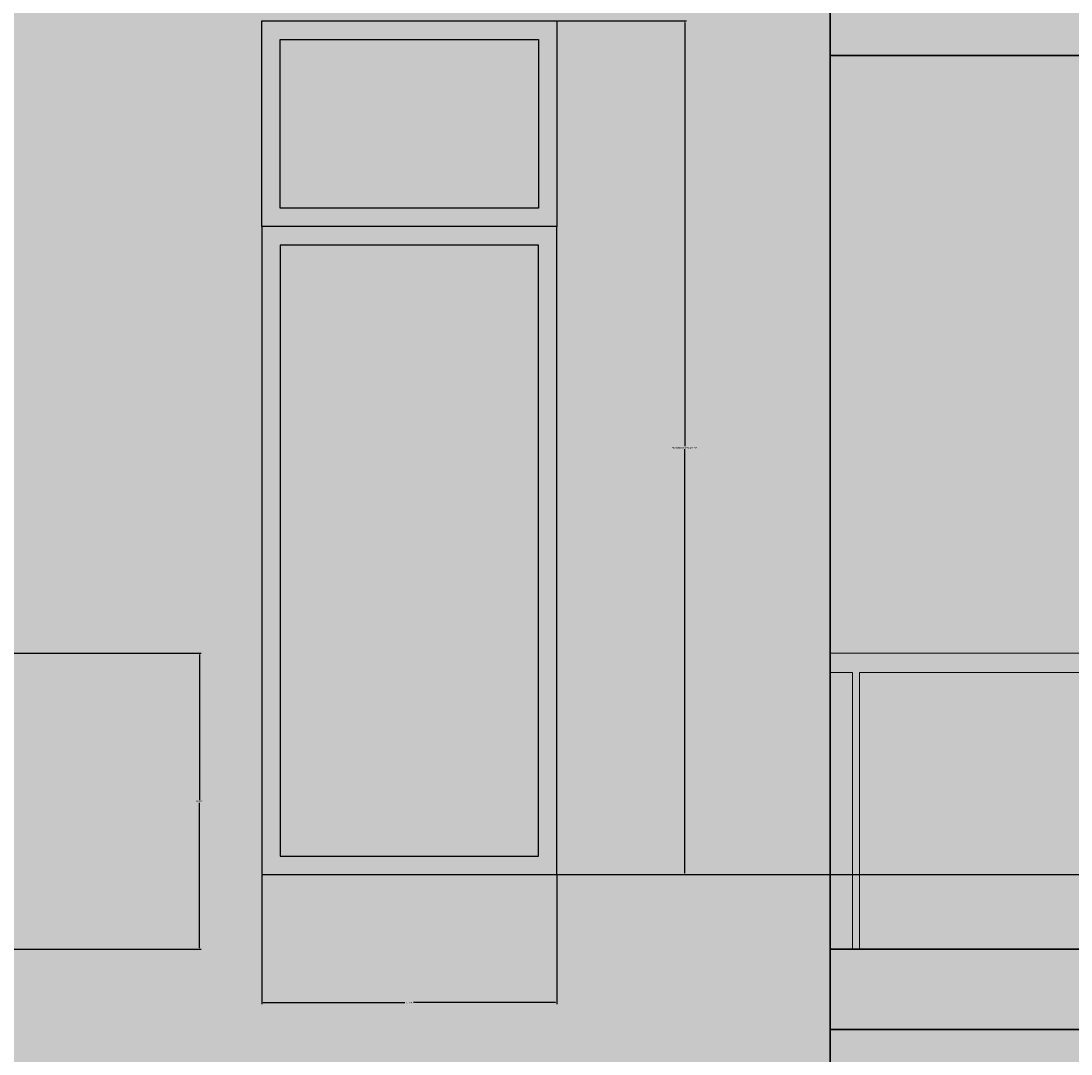
# Model space of a CAD drawing. Units: feet. Extents: x 2893 to 4112, y 897 to 1573.
# Tile 3 of 7: x 3123 to 3253, y 1090 to 1217. Entities that reach past the tile are written whole.
import ezdxf

# ---------------------------------------------------------------- set-up
doc = ezdxf.new("R2010")
doc.units = ezdxf.units.FT
for name, color, linetype, lineweight in [('A-ANNO-DIMS', 2, 'Continuous', 18), ('A-ELEV', 7, 'Continuous', 35), ('A-ELEV-PATT', 8, 'Continuous', 13), ('A-ELEV-RAIL', 4, 'Continuous', 18), ('A-GLAZ', 4, 'Continuous', 25)]:
    doc.layers.add(name, color=color, linetype=linetype, lineweight=lineweight)
doc.styles.get("Standard").update_dxf_attribs({"font": 'arial.ttf'})
doc.dimstyles.get("Standard").update_dxf_attribs({"dimtxt": 0.18, "dimasz": 0.18, "dimexe": 0.18, "dimexo": 0.0625, "dimgap": 0.09, "dimtad": 0, "dimtih": 1, "dimtoh": 1, "dimdec": 1, "dimzin": 0, "dimdsep": 46, "dimlunit": 3, "dimtxsty": 'Standard', "dimcen": 0.09, "dimadec": 0, "dimazin": 0, "dimtfac": 1, "dimtdec": 1, "dimtofl": 0, "dimtmove": 0, "dimatfit": 3, "dimfxl": 1, "dimtolj": 1, "dimtzin": 0, "dimarcsym": 0})

# ---------------------------------------------------------------- blocks, each defined once
blk = doc.blocks.new('WIN-FEATURE')
for points in [[(36.35, 79.81), (0, 79.81), (0, 105.14), (36.35, 105.14)], [(36.35, 79.81), (0, 79.81), (0, 105.14), (36.35, 105.14)], [(34.08, 82.08), (2.27, 82.08), (2.27, 102.87), (34.08, 102.87)], [(34.08, 82.08), (2.27, 82.08), (2.27, 102.87), (34.08, 102.87)], [(0, 0), (36.35, 0), (36.35, 79.81), (0, 79.81)], [(0, 0), (36.35, 0), (36.35, 79.81), (0, 79.81)], [(2.27, 2.27), (34.08, 2.27), (34.08, 77.54), (2.27, 77.54)], [(2.27, 2.27), (34.08, 2.27), (34.08, 77.54), (2.27, 77.54)]]:
    blk.add_lwpolyline(points, close=True)
blk = doc.blocks.new('BALCONY-RAIL')
blk.add_lwpolyline([(56.56, 34.07), (3.3, 34.07), (3.3, 0), (2.43, 0), (2.43, 34.07), (0, 34.07), (0, 36.45), (173.25, 36.45), (173.25, 34.07), (170.48, 34.07), (170.48, 0), (169.61, 0), (169.61, 34.07), (115.47, 34.07), (115.47, 0), (114.59, 0), (114.59, 34.07), (57.43, 34.07), (57.43, 0), (56.56, 0)], close=True)
blk.add_lwpolyline([(56.56, 34.07), (3.3, 34.07), (3.3, 0), (2.43, 0), (2.43, 34.07), (0, 34.07), (0, 36.45), (173.25, 36.45), (173.25, 34.07), (170.48, 34.07), (170.48, 0), (169.61, 0), (169.61, 34.07), (115.47, 34.07), (115.47, 0), (114.59, 0), (114.59, 34.07), (57.43, 34.07), (57.43, 0), (56.56, 0)], close=True)
blk = doc.blocks.new('*D8')
at = {"layer": 'A-ANNO-DIMS', "color": 0, "lineweight": -2, "transparency": 16777216}
for p, q in [((3119.39, 1139.38), (3145.49, 1139.38)), ((3145.31, 1139.2), (3145.31, 1121.34)), ((3145.31, 1103.11), (3145.31, 1120.97)), ((3119.39, 1102.93), (3145.49, 1102.93))]:
    blk.add_line(p, q, dxfattribs=at)
at = {"layer": 'A-ANNO-DIMS', "color": 0, "transparency": 16777216}
for points in [[(3145.28, 1139.2), (3145.34, 1139.2), (3145.31, 1139.38)], [(3145.28, 1103.11), (3145.34, 1103.11), (3145.31, 1102.93)]]:
    blk.add_solid(points, dxfattribs=at)
at = {"layer": 'Defpoints', "color": 0, "transparency": 16777216}
for p in [(3119.33, 1139.38), (3145.31, 1139.38), (3119.33, 1102.93)]:
    blk.add_point(p, dxfattribs=at)
at = {"layer": 'A-ANNO-DIMS', "color": 0, "transparency": 16777216, "insert": (3145.31, 1121.16), "char_height": 0.18, "attachment_point": 5}
blk.add_mtext('\\A1;36 TYP.', dxfattribs=at)
blk = doc.blocks.new('*D9')
at = {"layer": 'A-ANNO-DIMS', "color": 0, "lineweight": -2, "transparency": 16777216}
for p, q in [((3189.38, 1217.25), (3205.27, 1217.25)), ((3205.09, 1217.07), (3205.09, 1164.86)), ((3205.09, 1112.29), (3205.09, 1164.5)), ((3189.38, 1112.11), (3205.27, 1112.11))]:
    blk.add_line(p, q, dxfattribs=at)
at = {"layer": 'A-ANNO-DIMS', "color": 0, "transparency": 16777216}
for points in [[(3205.06, 1217.07), (3205.12, 1217.07), (3205.09, 1217.25)], [(3205.06, 1112.29), (3205.12, 1112.29), (3205.09, 1112.11)]]:
    blk.add_solid(points, dxfattribs=at)
at = {"layer": 'Defpoints', "color": 0, "transparency": 16777216}
for p in [(3189.32, 1217.25), (3205.09, 1217.25), (3189.32, 1112.11)]:
    blk.add_point(p, dxfattribs=at)
at = {"layer": 'A-ANNO-DIMS', "color": 0, "transparency": 16777216, "insert": (3205.09, 1164.68), "char_height": 0.18, "attachment_point": 5}
blk.add_mtext('\\A1;FEATURE WINDOW 105 TYP.', dxfattribs=at)
blk = doc.blocks.new('*D10')
at = {"layer": 'A-ANNO-DIMS', "color": 0, "lineweight": -2, "transparency": 16777216}
for p, q in [((3152.97, 1112.05), (3152.97, 1096.16)), ((3189.32, 1112.05), (3189.32, 1096.16)), ((3153.15, 1096.34), (3170.61, 1096.34)), ((3189.14, 1096.34), (3171.67, 1096.34))]:
    blk.add_line(p, q, dxfattribs=at)
at = {"layer": 'A-ANNO-DIMS', "color": 0, "transparency": 16777216}
for points in [[(3153.15, 1096.37), (3153.15, 1096.31), (3152.97, 1096.34)], [(3189.14, 1096.37), (3189.14, 1096.31), (3189.32, 1096.34)]]:
    blk.add_solid(points, dxfattribs=at)
at = {"layer": 'Defpoints', "color": 0, "transparency": 16777216}
for p in [(3152.97, 1112.11), (3189.32, 1112.11), (3189.32, 1096.34)]:
    blk.add_point(p, dxfattribs=at)
at = {"layer": 'A-ANNO-DIMS', "color": 0, "transparency": 16777216, "insert": (3171.14, 1096.34), "char_height": 0.18, "attachment_point": 5}
blk.add_mtext('\\A1;36 TYP.', dxfattribs=at)
blk = doc.blocks.new('*D48')
at = {"layer": 'A-ANNO-DIMS', "color": 0, "lineweight": -2, "transparency": 16777216}
for p, q in [((2924.72, 1491.83), (2924.72, 897.37)), ((3417.56, 1491.83), (3417.56, 897.37)), ((2924.9, 897.55), (3170.74, 897.55)), ((3417.38, 897.55), (3171.54, 897.55))]:
    blk.add_line(p, q, dxfattribs=at)
at = {"layer": 'A-ANNO-DIMS', "color": 0, "transparency": 16777216}
for points in [[(2924.9, 897.58), (2924.9, 897.52), (2924.72, 897.55)], [(3417.38, 897.58), (3417.38, 897.52), (3417.56, 897.55)]]:
    blk.add_solid(points, dxfattribs=at)
at = {"layer": 'Defpoints', "color": 0, "transparency": 16777216}
for p in [(2924.72, 1491.89), (3417.56, 1491.89), (3417.56, 897.55)]:
    blk.add_point(p, dxfattribs=at)
at = {"layer": 'A-ANNO-DIMS', "color": 0, "transparency": 16777216, "insert": (3171.14, 897.55), "char_height": 0.18, "attachment_point": 5}
blk.add_mtext('\\A1;492.8', dxfattribs=at)
blk = doc.blocks.new('*D51')
at = {"layer": 'A-ANNO-DIMS', "color": 0, "lineweight": -2, "transparency": 16777216}
for p, q in [((3189.38, 1112.11), (3449.24, 1112.11)), ((3449.06, 1111.93), (3449.06, 1099.74)), ((3449.06, 1087.19), (3449.06, 1099.38)), ((3215.03, 1087.01), (3449.24, 1087.01))]:
    blk.add_line(p, q, dxfattribs=at)
at = {"layer": 'A-ANNO-DIMS', "color": 0, "transparency": 16777216}
for points in [[(3449.03, 1111.93), (3449.09, 1111.93), (3449.06, 1112.11)], [(3449.03, 1087.19), (3449.09, 1087.19), (3449.06, 1087.01)]]:
    blk.add_solid(points, dxfattribs=at)
at = {"layer": 'Defpoints', "color": 0, "transparency": 16777216}
for p in [(3189.32, 1112.11), (3449.06, 1112.11), (3214.97, 1087.01)]:
    blk.add_point(p, dxfattribs=at)
at = {"layer": 'A-ANNO-DIMS', "color": 0, "transparency": 16777216, "insert": (3449.06, 1099.56), "char_height": 0.18, "attachment_point": 5}
blk.add_mtext('\\A1;25.095', dxfattribs=at)

msp = doc.modelspace()

# ---------------------------------------------------------------- hatches: boundary and pattern name
at = {"layer": 'A-ELEV-PATT'}
h = msp.add_hatch(color=256, dxfattribs=at)
h.dxf.hatch_style = 1
h.paths.add_polyline_path([(3222.9589, 1541.1646), (3119.3255, 1541.1646), (3119.3255, 967.0143), (3127.3151, 967.0143), (3127.3151, 1087.0143), (3214.9693, 1087.0143), (3214.9693, 1078.6766), (3214.9693, 967.0143), (3222.9589, 967.0143)])
h.paths.add_polyline_path([(3152.9675, 1482.3616), (3189.3169, 1482.3616), (3189.3169, 1457.0324), (3189.3169, 1377.2236), (3152.9675, 1377.2236), (3152.9675, 1457.0324)], flags=16)
h.paths.add_polyline_path([(3155.237, 1480.0922), (3187.0474, 1480.0922), (3187.0474, 1459.3019), (3155.237, 1459.3019)], flags=0)
h.paths.add_polyline_path([(3155.237, 1454.7629), (3187.0474, 1454.7629), (3187.0474, 1379.4931), (3155.237, 1379.4931)], flags=0)
h.paths.add_polyline_path([(3152.9675, 1354.8437), (3189.3169, 1354.8437), (3189.3169, 1329.5145), (3189.3169, 1249.7057), (3152.9675, 1249.7057), (3152.9675, 1329.5145)], flags=16)
h.paths.add_polyline_path([(3155.237, 1352.5742), (3187.0474, 1352.5742), (3187.0474, 1331.784), (3155.237, 1331.784)], flags=0)
h.paths.add_polyline_path([(3155.237, 1327.245), (3187.0474, 1327.245), (3187.0474, 1251.9752), (3155.237, 1251.9752)], flags=0)
h.paths.add_polyline_path([(3152.9675, 1217.2478), (3189.3169, 1217.2478), (3189.3169, 1191.9186), (3189.3169, 1112.1098), (3152.9675, 1112.1098), (3152.9675, 1191.9186)], flags=16)
h.paths.add_polyline_path([(3155.237, 1214.9783), (3187.0474, 1214.9783), (3187.0474, 1194.1881), (3155.237, 1194.1881)], flags=0)
h.paths.add_polyline_path([(3155.237, 1189.6491), (3187.0474, 1189.6491), (3187.0474, 1114.3793), (3155.237, 1114.3793)], flags=0)
h = msp.add_hatch(dxfattribs=at)
h.set_pattern_fill('AR-BRELM', color=256, scale=0.1)
h.set_pattern_definition([(0, (-663.002, 0), (0, 13.5484), [19.3675, -0.9525]), (0, (-663.002, 5.715), (0, 13.5484), [19.3675, -0.9525]), (0, (-657.922, 6.774), (0, 13.5484), [9.2075, -0.9525]), (0, (-657.922, 12.489), (0, 13.5484), [9.2075, -0.9525]), (90, (-663.002, 0), (-20.32, 1e-15), [5.715, -7.8334]), (90, (-663.954, 0), (-20.32, 1e-15), [5.715, -7.8334]), (90, (-657.922, 6.774), (-10.16, 6e-16), [5.715, -7.8334]), (90, (-658.874, 6.774), (-10.16, 6e-16), [5.715, -7.8334])])
h.paths.add_polyline_path([(3222.9589, 1541.1646), (3119.3255, 1541.1646), (3119.3255, 967.0143), (3127.3151, 967.0143), (3127.3151, 1087.0143), (3214.9693, 1087.0143), (3214.9693, 1078.6766), (3214.9693, 967.0143), (3222.9589, 967.0143)])
h.paths.add_polyline_path([(3152.9675, 1482.3616), (3189.3169, 1482.3616), (3189.3169, 1457.0324), (3189.3169, 1377.2236), (3152.9675, 1377.2236), (3152.9675, 1457.0324)], flags=16)
h.paths.add_polyline_path([(3155.237, 1480.0922), (3187.0474, 1480.0922), (3187.0474, 1459.3019), (3155.237, 1459.3019)], flags=0)
h.paths.add_polyline_path([(3155.237, 1454.7629), (3187.0474, 1454.7629), (3187.0474, 1379.4931), (3155.237, 1379.4931)], flags=0)
h.paths.add_polyline_path([(3152.9675, 1354.8437), (3189.3169, 1354.8437), (3189.3169, 1329.5145), (3189.3169, 1249.7057), (3152.9675, 1249.7057), (3152.9675, 1329.5145)], flags=16)
h.paths.add_polyline_path([(3155.237, 1352.5742), (3187.0474, 1352.5742), (3187.0474, 1331.784), (3155.237, 1331.784)], flags=0)
h.paths.add_polyline_path([(3155.237, 1327.245), (3187.0474, 1327.245), (3187.0474, 1251.9752), (3155.237, 1251.9752)], flags=0)
h.paths.add_polyline_path([(3152.9675, 1217.2478), (3189.3169, 1217.2478), (3189.3169, 1191.9186), (3189.3169, 1112.1098), (3152.9675, 1112.1098), (3152.9675, 1191.9186)], flags=16)
h.paths.add_polyline_path([(3155.237, 1214.9783), (3187.0474, 1214.9783), (3187.0474, 1194.1881), (3155.237, 1194.1881)], flags=0)
h.paths.add_polyline_path([(3155.237, 1189.6491), (3187.0474, 1189.6491), (3187.0474, 1114.3793), (3155.237, 1114.3793)], flags=0)
h = msp.add_hatch(color=256, dxfattribs=at)
h.dxf.hatch_style = 1
h.paths.add_polyline_path([(3119.3255, 1527.889), (2924.7207, 1527.889), (2924.7207, 1491.889), (3119.3255, 1491.889)])
h.paths.add_polyline_path([(3417.5637, 1527.889), (3222.9589, 1527.889), (3222.9589, 1491.889), (3417.5637, 1491.889)])
h.paths.add_polyline_path([(3119.3255, 1102.9302), (2946.0771, 1102.9302), (2946.0771, 1139.3799), (2934.0287, 1139.3799), (2934.0287, 1093.0143), (3119.3255, 1093.0143)])
h.paths.add_polyline_path([(3119.3255, 1093.0143), (2934.4679, 1093.0143), (2934.4679, 1087.0143), (3119.3255, 1087.0143)])
h.paths.add_polyline_path([(3408.2557, 1139.3799), (3396.2073, 1139.3799), (3396.2073, 1136.9984), (3396.2073, 1102.9302), (3222.9589, 1102.9302), (3222.9589, 1093.0143), (3408.2557, 1093.0143)])
h.paths.add_polyline_path([(3407.8165, 1093.0143), (3222.9589, 1093.0143), (3222.9589, 1087.0143), (3407.8165, 1087.0143)])
h = msp.add_hatch(color=256, dxfattribs=at)
h.dxf.hatch_style = 1
h.paths.add_polyline_path([(3119.3255, 1491.889), (2924.7207, 1491.889), (2945.7801, 1471.0143), (3119.3255, 1471.0143)])
h.paths.add_polyline_path([(3119.3255, 1471.0143), (2945.7801, 1471.0143), (2951.8333, 1465.0143), (3119.3255, 1465.0143)])
h.paths.add_polyline_path([(3119.3255, 1465.0143), (2951.8333, 1465.0143), (2951.8333, 1381.4641), (2984.02, 1381.4641), (2984.02, 1432.3761), (3084.4999, 1432.3761), (3084.4999, 1381.4641), (3119.3255, 1381.4641)])
h.paths.add_polyline_path([(3417.5637, 1491.889), (3222.9589, 1491.889), (3222.9589, 1471.0143), (3396.5042, 1471.0143)])
h.paths.add_polyline_path([(3396.5042, 1471.0143), (3222.9589, 1471.0143), (3222.9589, 1465.0143), (3390.4511, 1465.0143)])
h.paths.add_polyline_path([(3390.4511, 1465.0143), (3222.9589, 1465.0143), (3222.9589, 1381.4641), (3257.7845, 1381.4641), (3257.7845, 1432.3761), (3358.2644, 1432.3761), (3358.2644, 1381.4641), (3390.4511, 1381.4641)])
h.paths.add_polyline_path([(3119.3255, 1339.0143), (2942.6825, 1339.0143), (2942.6825, 1232.1197), (2948.5078, 1232.1197), (2948.5078, 1266.188), (2946.0771, 1266.188), (2946.0771, 1268.5695), (2984.02, 1268.5695), (2984.02, 1319.4815), (3084.4999, 1319.4815), (3084.4999, 1268.5695), (3119.3255, 1268.5695)], flags=17)
h.paths.add_polyline_path([(3399.6019, 1339.0143), (3222.9589, 1339.0143), (3222.9589, 1268.5695), (3257.7845, 1268.5695), (3257.7845, 1319.4815), (3358.2644, 1319.4815), (3358.2644, 1268.5695), (3396.2073, 1268.5695), (3396.2073, 1266.188), (3393.7766, 1266.188), (3393.7766, 1232.1197), (3399.6019, 1232.1197)], flags=17)
h.paths.add_polyline_path([(2942.6825, 1339.0143), (3119.3255, 1339.0143), (3119.3255, 1345.0143), (2933.3946, 1345.0143), (2933.3946, 1232.1197), (2933.3946, 1220.0947), (3119.3255, 1220.0947), (3119.3255, 1232.1197), (2942.6825, 1232.1197)])
h.paths.add_polyline_path([(3408.8898, 1345.0143), (3222.9589, 1345.0143), (3222.9589, 1339.0143), (3399.6019, 1339.0143), (3399.6019, 1232.1197), (3393.7766, 1232.1197), (3392.9028, 1232.1197), (3222.9589, 1232.1197), (3222.9589, 1220.0947), (3408.8898, 1220.0947), (3408.8898, 1232.1197)])
h.paths.add_polyline_path([(2984.02, 1190.2919), (3084.4999, 1190.2919), (3084.4999, 1139.3799), (3119.3255, 1139.3799), (3119.3255, 1213.0143), (2951.8333, 1213.0143), (2951.8333, 1139.3799), (2984.02, 1139.3799)])
h.paths.add_polyline_path([(3119.3255, 1219.0143), (2934.0287, 1219.0143), (2951.8333, 1213.0143), (3119.3255, 1213.0143)])
h.paths.add_polyline_path([(3390.4511, 1213.0143), (3222.9589, 1213.0143), (3222.9589, 1139.3799), (3257.7845, 1139.3799), (3257.7845, 1190.2919), (3358.2644, 1190.2919), (3358.2644, 1139.3799), (3390.4511, 1139.3799)])
h.paths.add_polyline_path([(3408.2557, 1219.0143), (3222.9589, 1219.0143), (3222.9589, 1213.0143), (3408.2557, 1213.0143)])
h = msp.add_hatch(color=256, dxfattribs=at)
h.dxf.hatch_style = 1
h.paths.add_polyline_path([(3119.3255, 1139.3799), (2946.0771, 1139.3799), (2946.0771, 1136.9984), (2948.5078, 1136.9984), (2948.5078, 1102.9302), (2949.3816, 1102.9302), (2949.3816, 1136.9984), (3002.6337, 1136.9984), (3002.6337, 1102.9302), (3003.5075, 1102.9302), (3003.5075, 1136.9984), (3060.6708, 1136.9984), (3060.6708, 1102.9302), (3061.5445, 1102.9302), (3061.5445, 1136.9984), (3115.685, 1136.9984), (3115.685, 1102.9302), (3116.5588, 1102.9302), (3116.5588, 1136.9984), (3119.3255, 1136.9984)])
h.paths.add_polyline_path([(2987.1701, 1187.1419), (3033.6877, 1187.1419), (3033.6877, 1139.3799), (3034.8322, 1139.3799), (3034.8322, 1187.1419), (3081.3499, 1187.1419), (3081.3499, 1139.3799), (3084.4999, 1139.3799), (3084.4999, 1190.2919), (2984.02, 1190.2919), (2984.02, 1139.3799), (2987.1701, 1139.3799)])
h.paths.add_polyline_path([(2987.1701, 1316.3314), (3033.6877, 1316.3314), (3033.6877, 1268.5695), (3034.8322, 1268.5695), (3034.8322, 1316.3314), (3081.3499, 1316.3314), (3081.3499, 1268.5695), (3084.4999, 1268.5695), (3084.4999, 1319.4815), (2984.02, 1319.4815), (2984.02, 1268.5695), (2987.1701, 1268.5695)])
h.paths.add_polyline_path([(3003.5075, 1266.188), (3060.6708, 1266.188), (3060.6708, 1232.1197), (3061.5445, 1232.1197), (3061.5445, 1266.188), (3115.685, 1266.188), (3115.685, 1232.1197), (3116.5588, 1232.1197), (3116.5588, 1266.188), (3119.3255, 1266.188), (3119.3255, 1268.5695), (2946.0771, 1268.5695), (2946.0771, 1266.188), (2948.5078, 1266.188), (2948.5078, 1232.1197), (2949.3816, 1232.1197), (2949.3816, 1266.188), (3002.6337, 1266.188), (3002.6337, 1232.1197), (3003.5075, 1232.1197)])
h.paths.add_polyline_path([(2987.1701, 1429.226), (3033.6877, 1429.226), (3033.6877, 1381.4641), (3034.8322, 1381.4641), (3034.8322, 1429.226), (3081.3499, 1429.226), (3081.3499, 1381.4641), (3084.4999, 1381.4641), (3084.4999, 1432.3761), (2984.02, 1432.3761), (2984.02, 1381.4641), (2987.1701, 1381.4641)])
h.paths.add_polyline_path([(3119.3255, 1381.4641), (2946.0771, 1381.4641), (2946.0771, 1379.0826), (2948.5078, 1379.0826), (2948.5078, 1345.0143), (2949.3816, 1345.0143), (2949.3816, 1379.0826), (3002.6337, 1379.0826), (3002.6337, 1345.0143), (3003.5075, 1345.0143), (3003.5075, 1379.0826), (3060.6708, 1379.0826), (3060.6708, 1345.0143), (3061.5445, 1345.0143), (3061.5445, 1379.0826), (3115.685, 1379.0826), (3115.685, 1345.0143), (3116.5588, 1345.0143), (3116.5588, 1379.0826), (3119.3255, 1379.0826)])
h.paths.add_polyline_path([(3189.3169, 1482.3616), (3152.9675, 1482.3616), (3152.9675, 1457.0324), (3189.3169, 1457.0324)])
h.paths.add_polyline_path([(3155.237, 1480.0922), (3187.0474, 1480.0922), (3187.0474, 1459.3019), (3155.237, 1459.3019)], flags=16)
h.paths.add_polyline_path([(3189.3169, 1457.0324), (3152.9675, 1457.0324), (3152.9675, 1377.2236), (3189.3169, 1377.2236)])
h.paths.add_polyline_path([(3155.237, 1454.7629), (3187.0474, 1454.7629), (3187.0474, 1379.4931), (3155.237, 1379.4931)], flags=16)
h.paths.add_polyline_path([(3358.2644, 1432.3761), (3257.7845, 1432.3761), (3257.7845, 1381.4641), (3260.9345, 1381.4641), (3260.9345, 1429.226), (3307.4522, 1429.226), (3307.4522, 1381.4641), (3308.5967, 1381.4641), (3308.5967, 1429.226), (3355.1143, 1429.226), (3355.1143, 1381.4641), (3358.2644, 1381.4641)])
h.paths.add_polyline_path([(3396.2073, 1381.4641), (3222.9589, 1381.4641), (3222.9589, 1379.0826), (3225.7256, 1379.0826), (3225.7256, 1345.0143), (3226.5994, 1345.0143), (3226.5994, 1379.0826), (3280.7398, 1379.0826), (3280.7398, 1345.0143), (3281.6136, 1345.0143), (3281.6136, 1379.0826), (3338.7769, 1379.0826), (3338.7769, 1345.0143), (3339.6507, 1345.0143), (3339.6507, 1379.0826), (3392.9028, 1379.0826), (3392.9028, 1345.0143), (3393.7766, 1345.0143), (3393.7766, 1379.0826), (3396.2073, 1379.0826)])
h.paths.add_polyline_path([(3358.2644, 1319.4815), (3257.7845, 1319.4815), (3257.7845, 1268.5695), (3260.9345, 1268.5695), (3260.9345, 1316.3314), (3307.4522, 1316.3314), (3307.4522, 1268.5695), (3308.5967, 1268.5695), (3308.5967, 1316.3314), (3355.1143, 1316.3314), (3355.1143, 1268.5695), (3358.2644, 1268.5695)])
h.paths.add_polyline_path([(3396.2073, 1268.5695), (3222.9589, 1268.5695), (3222.9589, 1266.188), (3225.7256, 1266.188), (3225.7256, 1232.1197), (3226.5994, 1232.1197), (3226.5994, 1266.188), (3280.7398, 1266.188), (3280.7398, 1232.1197), (3281.6136, 1232.1197), (3281.6136, 1266.188), (3338.7769, 1266.188), (3338.7769, 1232.1197), (3339.6507, 1232.1197), (3339.6507, 1266.188), (3392.9028, 1266.188), (3392.9028, 1232.1197), (3393.7766, 1232.1197), (3393.7766, 1266.188), (3396.2073, 1266.188)])
h.paths.add_polyline_path([(3260.9345, 1187.1419), (3307.4522, 1187.1419), (3307.4522, 1139.3799), (3308.5967, 1139.3799), (3308.5967, 1187.1419), (3355.1143, 1187.1419), (3355.1143, 1139.3799), (3358.2644, 1139.3799), (3358.2644, 1190.2919), (3257.7845, 1190.2919), (3257.7845, 1139.3799), (3260.9345, 1139.3799)])
h.paths.add_polyline_path([(3396.2073, 1139.3799), (3222.9589, 1139.3799), (3222.9589, 1136.9984), (3225.7256, 1136.9984), (3225.7256, 1102.9302), (3226.5994, 1102.9302), (3226.5994, 1136.9984), (3280.7398, 1136.9984), (3280.7398, 1102.9302), (3281.6136, 1102.9302), (3281.6136, 1136.9984), (3338.7769, 1136.9984), (3338.7769, 1102.9302), (3339.6507, 1102.9302), (3339.6507, 1136.9984), (3392.9028, 1136.9984), (3392.9028, 1102.9302), (3393.7766, 1102.9302), (3393.7766, 1136.9984), (3396.2073, 1136.9984)])
h.paths.add_polyline_path([(3189.3169, 1354.8437), (3152.9675, 1354.8437), (3152.9675, 1329.5145), (3189.3169, 1329.5145)])
h.paths.add_polyline_path([(3155.237, 1331.784), (3155.237, 1352.5742), (3187.0474, 1352.5742), (3187.0474, 1331.784)], flags=16)
h.paths.add_polyline_path([(3189.3169, 1329.5145), (3152.9675, 1329.5145), (3152.9675, 1249.7057), (3189.3169, 1249.7057)])
h.paths.add_polyline_path([(3155.237, 1327.245), (3187.0474, 1327.245), (3187.0474, 1251.9752), (3155.237, 1251.9752)], flags=16)
h.paths.add_polyline_path([(3189.3169, 1191.9186), (3152.9675, 1191.9186), (3152.9675, 1112.1098), (3189.3169, 1112.1098)])
h.paths.add_polyline_path([(3155.237, 1189.6491), (3187.0474, 1189.6491), (3187.0474, 1114.3793), (3155.237, 1114.3793)], flags=16)
h.paths.add_polyline_path([(3189.3169, 1217.2478), (3152.9675, 1217.2478), (3152.9675, 1191.9186), (3189.3169, 1191.9186)])
h.paths.add_polyline_path([(3155.237, 1194.1881), (3155.237, 1214.9783), (3187.0474, 1214.9783), (3187.0474, 1194.1881)], flags=16)
h = msp.add_hatch(color=256, dxfattribs=at)
h.dxf.hatch_style = 1
h.paths.add_polyline_path([(3033.6877, 1429.226), (2987.1701, 1429.226), (2987.1701, 1381.4641), (3033.6877, 1381.4641)])
h.paths.add_polyline_path([(3081.3499, 1429.226), (3034.8322, 1429.226), (3034.8322, 1381.4641), (3081.3499, 1381.4641)])
h.paths.add_polyline_path([(3115.685, 1379.0826), (3061.5445, 1379.0826), (3061.5445, 1345.0143), (3115.685, 1345.0143)])
h.paths.add_polyline_path([(3119.3255, 1379.0826), (3116.5588, 1379.0826), (3116.5588, 1345.0143), (3119.3255, 1345.0143)])
h.paths.add_polyline_path([(3060.6708, 1379.0826), (3003.5075, 1379.0826), (3003.5075, 1345.0143), (3060.6708, 1345.0143)])
h.paths.add_polyline_path([(3002.6337, 1379.0826), (2949.3816, 1379.0826), (2949.3816, 1345.0143), (3002.6337, 1345.0143)])
h.paths.add_polyline_path([(2948.5078, 1379.0826), (2946.0771, 1379.0826), (2946.0771, 1345.0143), (2948.5078, 1345.0143)])
h.paths.add_polyline_path([(3355.1143, 1429.226), (3308.5967, 1429.226), (3308.5967, 1381.4641), (3355.1143, 1381.4641)])
h.paths.add_polyline_path([(3307.4522, 1429.226), (3260.9345, 1429.226), (3260.9345, 1381.4641), (3307.4522, 1381.4641)])
h.paths.add_polyline_path([(3225.7256, 1379.0826), (3222.9589, 1379.0826), (3222.9589, 1345.0143), (3225.7256, 1345.0143)])
h.paths.add_polyline_path([(3280.7398, 1379.0826), (3226.5994, 1379.0826), (3226.5994, 1345.0143), (3280.7398, 1345.0143)])
h.paths.add_polyline_path([(3338.7769, 1379.0826), (3281.6136, 1379.0826), (3281.6136, 1345.0143), (3338.7769, 1345.0143)])
h.paths.add_polyline_path([(3392.9028, 1379.0826), (3339.6507, 1379.0826), (3339.6507, 1345.0143), (3392.9028, 1345.0143)])
h.paths.add_polyline_path([(3187.0474, 1480.0922), (3155.237, 1480.0922), (3155.237, 1459.3019), (3187.0474, 1459.3019)])
h.paths.add_polyline_path([(3187.0474, 1454.7629), (3155.237, 1454.7629), (3155.237, 1379.4931), (3187.0474, 1379.4931)])
h.paths.add_polyline_path([(3187.0474, 1352.5742), (3155.237, 1352.5742), (3155.237, 1331.784), (3187.0474, 1331.784)])
h.paths.add_polyline_path([(3187.0474, 1327.245), (3155.237, 1327.245), (3155.237, 1251.9752), (3187.0474, 1251.9752)])
h.paths.add_polyline_path([(3033.6877, 1316.3314), (2987.1701, 1316.3314), (2987.1701, 1268.5695), (3033.6877, 1268.5695)])
h.paths.add_polyline_path([(3081.3499, 1316.3314), (3034.8322, 1316.3314), (3034.8322, 1268.5695), (3081.3499, 1268.5695)])
h.paths.add_polyline_path([(3002.6337, 1266.188), (2949.3816, 1266.188), (2949.3816, 1232.1197), (3002.6337, 1232.1197)])
h.paths.add_polyline_path([(3060.6708, 1266.188), (3003.5075, 1266.188), (3003.5075, 1232.1197), (3060.6708, 1232.1197)])
h.paths.add_polyline_path([(3115.685, 1266.188), (3061.5445, 1266.188), (3061.5445, 1232.1197), (3115.685, 1232.1197)])
h.paths.add_polyline_path([(3119.3255, 1266.188), (3116.5588, 1266.188), (3116.5588, 1232.1197), (3119.3255, 1232.1197)])
h.paths.add_polyline_path([(3307.4522, 1316.3314), (3260.9345, 1316.3314), (3260.9345, 1268.5695), (3307.4522, 1268.5695)])
h.paths.add_polyline_path([(3355.1143, 1316.3314), (3308.5967, 1316.3314), (3308.5967, 1268.5695), (3355.1143, 1268.5695)])
h.paths.add_polyline_path([(3392.9028, 1266.188), (3339.6507, 1266.188), (3339.6507, 1232.1197), (3392.9028, 1232.1197)])
h.paths.add_polyline_path([(3338.7769, 1266.188), (3281.6136, 1266.188), (3281.6136, 1232.1197), (3338.7769, 1232.1197)])
h.paths.add_polyline_path([(3280.7398, 1266.188), (3226.5994, 1266.188), (3226.5994, 1232.1197), (3280.7398, 1232.1197)])
h.paths.add_polyline_path([(3225.7256, 1266.188), (3222.9589, 1266.188), (3222.9589, 1232.1197), (3225.7256, 1232.1197)])
h.paths.add_polyline_path([(3033.6877, 1187.1419), (2987.1701, 1187.1419), (2987.1701, 1139.3799), (3033.6877, 1139.3799)])
h.paths.add_polyline_path([(3081.3499, 1187.1419), (3034.8322, 1187.1419), (3034.8322, 1139.3799), (3081.3499, 1139.3799)])
h.paths.add_polyline_path([(3002.6337, 1136.9984), (2949.3816, 1136.9984), (2949.3816, 1102.9302), (3002.6337, 1102.9302)])
h.paths.add_polyline_path([(3060.6708, 1136.9984), (3003.5075, 1136.9984), (3003.5075, 1102.9302), (3060.6708, 1102.9302)])
h.paths.add_polyline_path([(3115.685, 1136.9984), (3061.5445, 1136.9984), (3061.5445, 1102.9302), (3115.685, 1102.9302)])
h.paths.add_polyline_path([(3187.0474, 1214.9783), (3155.237, 1214.9783), (3155.237, 1194.1881), (3187.0474, 1194.1881)])
h.paths.add_polyline_path([(3187.0474, 1189.6491), (3155.237, 1189.6491), (3155.237, 1114.3793), (3187.0474, 1114.3793)])
h.paths.add_polyline_path([(3307.4522, 1187.1419), (3260.9345, 1187.1419), (3260.9345, 1139.3799), (3307.4522, 1139.3799)])
h.paths.add_polyline_path([(3355.1143, 1187.1419), (3308.5967, 1187.1419), (3308.5967, 1139.3799), (3355.1143, 1139.3799)])
h.paths.add_polyline_path([(3280.7398, 1136.9984), (3226.5994, 1136.9984), (3226.5994, 1102.9302), (3280.7398, 1102.9302)])
h.paths.add_polyline_path([(3338.7769, 1136.9984), (3281.6136, 1136.9984), (3281.6136, 1102.9302), (3338.7769, 1102.9302)])
h.paths.add_polyline_path([(3392.9028, 1136.9984), (3339.6507, 1136.9984), (3339.6507, 1102.9302), (3392.9028, 1102.9302)])
h.paths.add_polyline_path([(3225.7256, 1136.9984), (3222.9589, 1136.9984), (3222.9589, 1102.9302), (3225.7256, 1102.9302)])
h.paths.add_polyline_path([(3119.3255, 1136.9984), (3116.5588, 1136.9984), (3116.5588, 1102.9302), (3119.3255, 1102.9302)])
h.paths.add_polyline_path([(2948.5078, 1136.9984), (2946.0771, 1136.9984), (2946.0771, 1102.9302), (2948.5078, 1102.9302)])
h.paths.add_polyline_path([(3396.2073, 1136.9984), (3393.7766, 1136.9984), (3393.7766, 1102.9302), (3396.2073, 1102.9302)])

# ---------------------------------------------------------------- linework, layer by layer
at = {"layer": 'A-ELEV'}
for p, q in [((3222.9589, 967.0143), (3222.9589, 1541.1646)), ((3222.9589, 1213.0143), (3408.2557, 1213.0143)), ((3222.9589, 1213.0143), (3408.2557, 1213.0143)), ((3222.9589, 1093.0143), (3408.2557, 1093.0143))]:
    msp.add_line(p, q, dxfattribs=at)
for points in [[(3119.3255, 967.0143), (3119.3255, 1541.1646), (3222.9589, 1541.1646), (3222.9589, 967.0143)], [(3222.9589, 1093.0143), (3408.2557, 1093.0143), (3408.2557, 1139.3799), (3396.2073, 1139.3799), (3396.2073, 1102.9302), (3222.9589, 1102.9302), (3222.9589, 1087.0143), (3407.8165, 1087.0143), (3407.8165, 1093.0143)], [(3222.9589, 1087.0143), (3222.9589, 1102.9302), (3396.2073, 1102.9302)]]:
    msp.add_lwpolyline(points, dxfattribs=at)

# ---------------------------------------------------------------- block references
at = {"layer": 'A-ELEV-RAIL', "extrusion": (0, 0, -1), "zscale": -1}
msp.add_blockref('BALCONY-RAIL', (-3396.2074, 1102.93), dxfattribs=at)
at = {"layer": 'A-GLAZ'}
msp.add_blockref('WIN-FEATURE', (3152.967, 1112.11), dxfattribs=at)

# ---------------------------------------------------------------- dimensions: what is measured, and where the dimension line sits
at = {"layer": 'A-ANNO-DIMS'}
dim = msp.add_linear_dim(base=(3417.5637, 897.5499), p1=(2924.7207, 1491.889), p2=(3417.5637, 1491.889), dimstyle='Standard', override={"dimdec": 1, "dimlfac": 1, "dimrnd": 0, "dimzin": 0, "dimdsep": 46, "dimlunit": 2}, dxfattribs=at)
dim.commit()
dim.dimension.update_dxf_attribs({"geometry": '*D48', "text_midpoint": (3171.1422, 897.5499)})
for base, p1, p2, text, picture, middle in [((3205.0876, 1217.2478), (3189.3169, 1112.1098), (3189.3169, 1217.2478), 'FEATURE WINDOW <> TYP.', '*D9', (3205.0876, 1164.6788)), ((3145.3128, 1139.3799), (3119.3255, 1102.9302), (3119.3255, 1139.3799), '<> TYP.', '*D8', (3145.3128, 1121.1551))]:
    dim = msp.add_linear_dim(base=base, p1=p1, p2=p2, angle=90, text=text, dimstyle='Standard', override={"dimdec": 0, "dimlfac": 1, "dimrnd": 0, "dimzin": 0, "dimdsep": 46, "dimlunit": 2}, dxfattribs=at)
    dim.commit()
    dim.dimension.update_dxf_attribs({"geometry": picture, "text_midpoint": middle})
dim = msp.add_linear_dim(base=(3189.3169, 1096.3391), p1=(3152.9675, 1112.1098), p2=(3189.3169, 1112.1098), text='<> TYP.', dimstyle='Standard', override={"dimdec": 0, "dimlfac": 1, "dimrnd": 0, "dimzin": 0, "dimdsep": 46, "dimlunit": 2}, dxfattribs=at)
dim.commit()
dim.dimension.update_dxf_attribs({"geometry": '*D10', "text_midpoint": (3171.1422, 1096.3391)})
dim = msp.add_linear_dim(base=(3449.06374, 1112.1098), p1=(3214.96934, 1087.01433), p2=(3189.3169, 1112.1098), angle=90, dimstyle='Standard', override={"dimdec": 3, "dimlfac": 1, "dimrnd": 0, "dimzin": 0, "dimdsep": 46, "dimlunit": 2}, dxfattribs=at)
dim.commit()
dim.dimension.update_dxf_attribs({"geometry": '*D51', "text_midpoint": (3449.06374, 1099.56206)})

doc.saveas('drawing.dxf')
